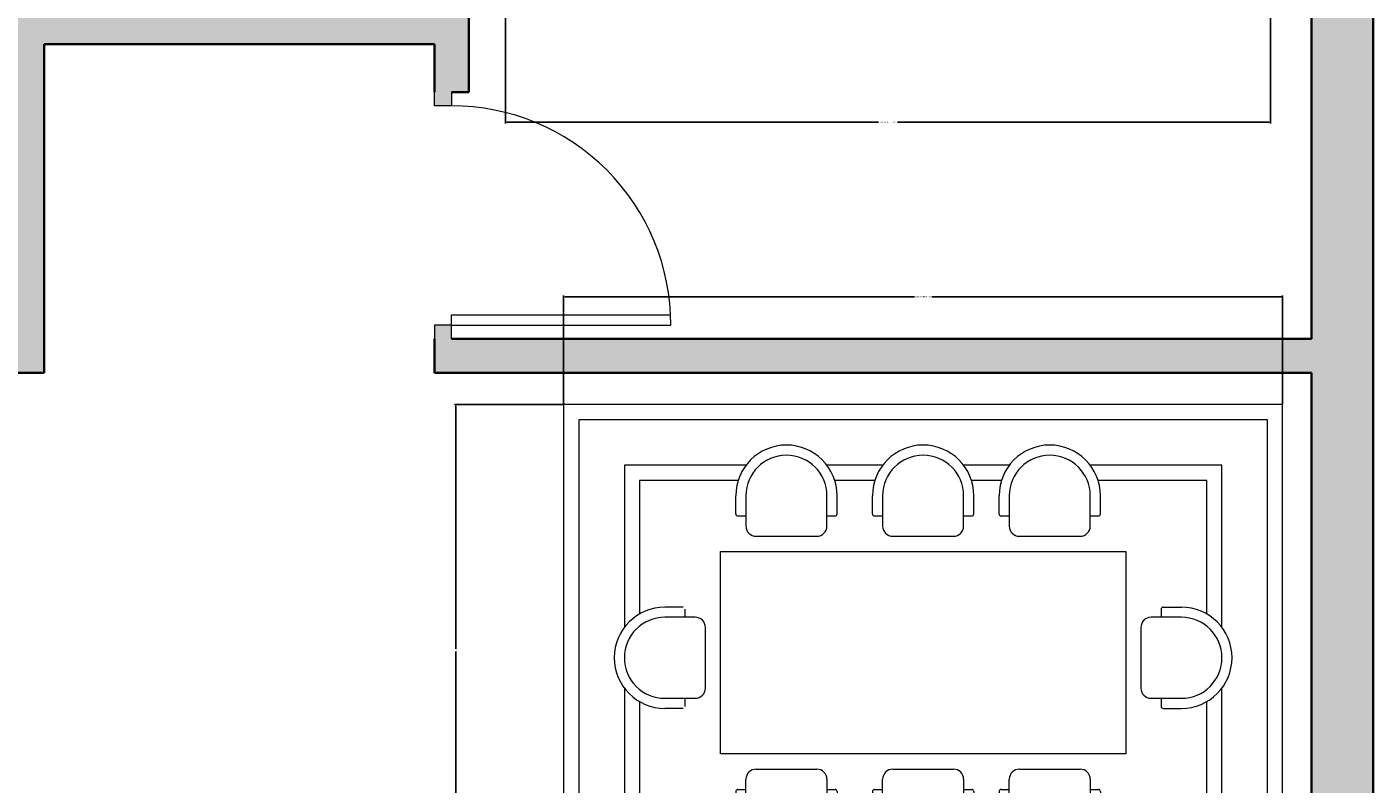
# Model space of a CAD drawing. Units: inches. Extents: x 2948 to 4025, y 2171 to 2966.
# Tile 4 of 6: x 3159 to 3356, y 2560 to 2670. Entities that reach past the tile are written whole.
import ezdxf

# ---------------------------------------------------------------- set-up
doc = ezdxf.new("R2010")
doc.units = ezdxf.units.IN
for name, color, linetype, lineweight in [('A-ANNO-DIMS', 2, 'Continuous', 18), ('A-DOOR', 3, 'Continuous', 18), ('A-FURN', 8, 'Continuous', 18), ('A-WALL', 7, 'Continuous', 35), ('A-WALL-PATT', 252, 'Continuous', 13)]:
    doc.layers.add(name, color=color, linetype=linetype, lineweight=lineweight)
doc.styles.get("Standard").update_dxf_attribs({"font": 'arial.ttf'})
doc.dimstyles.get("Standard").update_dxf_attribs({"dimtxt": 0.18, "dimasz": 0.18, "dimexe": 0.18, "dimexo": 0.0625, "dimgap": 0.09, "dimtad": 0, "dimtih": 1, "dimtoh": 1, "dimdec": 4, "dimzin": 0, "dimdsep": 46, "dimtxsty": 'Standard', "dimcen": 0.09, "dimadec": 0, "dimazin": 0, "dimtfac": 1, "dimtdec": 4, "dimtofl": 0, "dimtmove": 0, "dimatfit": 3, "dimfxl": 1, "dimtolj": 1, "dimtzin": 0, "dimarcsym": 0})

# ---------------------------------------------------------------- blocks, each defined once
blk = doc.blocks.new('A$C27801A2F')
for p, q in [((3.55, 2.425), (0, 2.425)), ((0, 2.425), (0, 0)), ((3.55, 0), (3.55, 2.425)), ((3.475, 2.35), (0.075, 2.35)), ((0.075, 2.35), (0.075, 0.075)), ((3.475, 0.075), (3.475, 2.35)), ((0.9, 2.125), (0.3, 2.125)), ((0.3, 2.125), (0.3, 1.325)), ((1.575, 2.125), (1.3, 2.125)), ((2.2, 2.125), (1.975, 2.125)), ((3.25, 2.125), (2.6, 2.125)), ((3.25, 1.325), (3.25, 2.125)), ((0.375, 2.05), (0.375, 1.3915)), ((0.8615, 2.05), (0.375, 2.05)), ((1.5365, 2.05), (1.3385, 2.05)), ((2.1615, 2.05), (2.0135, 2.05)), ((3.175, 2.05), (2.6385, 2.05)), ((3.175, 1.3915), (3.175, 2.05)), ((0.85, 1.885), (0.85, 1.975)), ((0.9, 1.975), (0.9, 1.825)), ((1.3, 1.825), (1.3, 1.975)), ((1.35, 1.885), (1.35, 1.975)), ((1.525, 1.885), (1.525, 1.975)), ((1.575, 1.975), (1.575, 1.825)), ((1.975, 1.825), (1.975, 1.975)), ((2.025, 1.885), (2.025, 1.975)), ((2.15, 1.885), (2.15, 1.975)), ((2.2, 1.975), (2.2, 1.825)), ((2.6, 1.825), (2.6, 1.975)), ((2.65, 1.885), (2.65, 1.975)), ((0.86, 1.875), (0.9, 1.875)), ((1.3, 1.875), (1.34, 1.875)), ((1.535, 1.875), (1.575, 1.875)), ((1.975, 1.875), (2.015, 1.875)), ((2.16, 1.875), (2.2, 1.875)), ((2.6, 1.875), (2.64, 1.875)), ((0.95, 1.775), (1.25, 1.775)), ((1.625, 1.775), (1.925, 1.775)), ((2.25, 1.775), (2.55, 1.775)), ((0.775, 0.7), (0.775, 1.7)), ((0.775, 1.7), (2.775, 1.7)), ((2.775, 1.7), (2.775, 0.7)), ((0.59, 1.425), (0.5, 1.425)), ((0.6, 1.375), (0.6, 1.415)), ((2.95, 1.415), (2.95, 1.375)), ((2.96, 1.425), (3.05, 1.425)), ((0.65, 1.375), (0.5, 1.375)), ((3.05, 1.375), (2.9, 1.375)), ((0.7, 1.025), (0.7, 1.325)), ((2.85, 1.325), (2.85, 1.025)), ((0.3, 1.025), (0.3, 0.275)), ((3.25, 0.275), (3.25, 1.025)), ((0.375, 0.9585), (0.375, 0.35)), ((0.5, 0.975), (0.65, 0.975)), ((0.6, 0.935), (0.6, 0.975)), ((2.9, 0.975), (3.05, 0.975)), ((2.95, 0.975), (2.95, 0.935)), ((3.175, 0.35), (3.175, 0.9585)), ((0.59, 0.925), (0.5, 0.925)), ((2.96, 0.925), (3.05, 0.925)), ((2.775, 0.7), (0.775, 0.7)), ((0.95, 0.625), (1.25, 0.625)), ((1.625, 0.625), (1.925, 0.625)), ((2.25, 0.625), (2.55, 0.625)), ((0.9, 0.425), (0.9, 0.575)), ((1.3, 0.575), (1.3, 0.425)), ((1.575, 0.425), (1.575, 0.575)), ((1.975, 0.575), (1.975, 0.425)), ((2.2, 0.425), (2.2, 0.575)), ((2.6, 0.575), (2.6, 0.425)), ((0.85, 0.515), (0.85, 0.425)), ((0.86, 0.525), (0.9, 0.525)), ((1.3, 0.525), (1.34, 0.525)), ((1.35, 0.515), (1.35, 0.425)), ((1.525, 0.515), (1.525, 0.425)), ((1.535, 0.525), (1.575, 0.525)), ((1.975, 0.525), (2.015, 0.525)), ((2.025, 0.515), (2.025, 0.425)), ((2.15, 0.515), (2.15, 0.425)), ((2.16, 0.525), (2.2, 0.525)), ((2.6, 0.525), (2.64, 0.525)), ((2.65, 0.515), (2.65, 0.425)), ((0.375, 0.35), (0.8615, 0.35)), ((1.3385, 0.35), (1.5365, 0.35)), ((2.0135, 0.35), (2.1615, 0.35)), ((2.6385, 0.35), (3.175, 0.35)), ((0.3, 0.275), (0.9, 0.275)), ((1.3, 0.275), (1.575, 0.275)), ((1.975, 0.275), (2.2, 0.275)), ((2.6, 0.275), (3.25, 0.275)), ((0.075, 0.075), (3.475, 0.075)), ((0, 0), (3.55, 0))]:
    blk.add_line(p, q)
for centre, radius, start, end in [((1.1, 1.975), 0.25, 0, 180), ((1.775, 1.975), 0.25, 0, 180), ((2.4, 1.975), 0.25, 0, 180), ((1.1, 1.975), 0.2, 0.00007, 179.99993), ((1.775, 1.975), 0.2, 0.00007, 179.99993), ((2.4, 1.975), 0.2, 0.00007, 179.99993), ((0.86, 1.885), 0.01, 180, 270), ((1.34, 1.885), 0.01, 270, 0), ((1.535, 1.885), 0.01, 180, 270), ((2.015, 1.885), 0.01, 270, 0), ((2.16, 1.885), 0.01, 180, 270), ((2.64, 1.885), 0.01, 270, 0), ((0.95, 1.825), 0.05, 180, 270), ((1.25, 1.825), 0.05, 270, 0), ((1.625, 1.825), 0.05, 180, 270), ((1.925, 1.825), 0.05, 270, 0), ((2.25, 1.825), 0.05, 180, 270), ((2.55, 1.825), 0.05, 270, 0), ((0.5, 1.175), 0.25, 90, 270), ((2.96, 1.415), 0.01, 90, 180), ((3.05, 1.175), 0.25, 270, 90), ((0.5, 1.175), 0.2, 90.00007, 269.99993), ((0.65, 1.325), 0.05, 0, 90), ((2.9, 1.325), 0.05, 90, 180), ((3.05, 1.175), 0.2, 270.00007, 89.99993), ((0.65, 1.025), 0.05, 270, 0), ((2.9, 1.025), 0.05, 180, 270), ((2.96, 0.935), 0.01, 180, 270), ((0.95, 0.575), 0.05, 90, 180), ((1.25, 0.575), 0.05, 0, 90), ((1.625, 0.575), 0.05, 90, 180), ((1.925, 0.575), 0.05, 0, 90), ((2.25, 0.575), 0.05, 90, 180), ((2.55, 0.575), 0.05, 0, 90), ((0.86, 0.515), 0.01, 90, 180), ((1.34, 0.515), 0.01, 0, 90), ((1.535, 0.515), 0.01, 90, 180), ((2.015, 0.515), 0.01, 0, 90), ((2.16, 0.515), 0.01, 90, 180), ((2.64, 0.515), 0.01, 0, 90), ((1.1, 0.425), 0.25, 180, 0), ((1.1, 0.425), 0.2, 180.00007, 359.99993), ((1.775, 0.425), 0.25, 180, 0), ((1.775, 0.425), 0.2, 180.00007, 359.99993), ((2.4, 0.425), 0.25, 180, 0), ((2.4, 0.425), 0.2, 180.00007, 359.99993)]:
    blk.add_arc(centre, radius, start, end)
blk = doc.blocks.new('DOOR-SWING-32IN')
for p, q in [((2, 34.5), (0, 34.5)), ((2, 32), (2, 34.5)), ((34, 32), (34, 34.5)), ((34, 34.5), (36, 34.5)), ((0, 32), (2, 32)), ((2, 32), (2, 0)), ((2, 32), (3.5, 32)), ((3.5, 32), (3.5, 0.04)), ((36, 32), (34, 32))]:
    blk.add_line(p, q)
blk.add_arc((2, 32), 32, 270, 0)
blk = doc.blocks.new('*D27')
at = {"layer": 'A-ANNO-DIMS', "color": 0, "lineweight": -2, "transparency": 16777216}
for p, q in [((3228.87, 2673.27), (3228.87, 2656.41)), ((3340.53, 2673.27), (3340.53, 2656.41)), ((3229.05, 2656.59), (3283.31, 2656.59)), ((3340.35, 2656.59), (3286.08, 2656.59))]:
    blk.add_line(p, q, dxfattribs=at)
at = {"layer": 'A-ANNO-DIMS', "color": 0, "transparency": 16777216}
for points in [[(3229.05, 2656.62), (3229.05, 2656.56), (3228.87, 2656.59)], [(3340.35, 2656.62), (3340.35, 2656.56), (3340.53, 2656.59)]]:
    blk.add_solid(points, dxfattribs=at)
at = {"layer": 'Defpoints', "color": 0, "transparency": 16777216}
for p in [(3228.87, 2673.34), (3340.53, 2673.34), (3340.53, 2656.59)]:
    blk.add_point(p, dxfattribs=at)
at = {"layer": 'A-ANNO-DIMS', "color": 0, "transparency": 16777216, "insert": (3284.7, 2656.59), "char_height": 0.18, "attachment_point": 5}
blk.add_mtext('\\A1;BED GROUP 112 TYP.', dxfattribs=at)
blk = doc.blocks.new('*D29')
at = {"layer": 'A-ANNO-DIMS', "color": 0, "lineweight": -2, "transparency": 16777216}
for p, q in [((3237.36, 2615.44), (3237.36, 2631.3)), ((3342.31, 2615.44), (3342.31, 2631.3)), ((3237.54, 2631.12), (3288.58, 2631.12)), ((3342.13, 2631.12), (3291.09, 2631.12))]:
    blk.add_line(p, q, dxfattribs=at)
at = {"layer": 'A-ANNO-DIMS', "color": 0, "transparency": 16777216}
for points in [[(3237.54, 2631.15), (3237.54, 2631.09), (3237.36, 2631.12)], [(3342.13, 2631.15), (3342.13, 2631.09), (3342.31, 2631.12)]]:
    blk.add_solid(points, dxfattribs=at)
at = {"layer": 'Defpoints', "color": 0, "transparency": 16777216}
for p in [(3342.31, 2631.12), (3237.36, 2615.38), (3342.31, 2615.38)]:
    blk.add_point(p, dxfattribs=at)
at = {"layer": 'A-ANNO-DIMS', "color": 0, "transparency": 16777216, "insert": (3289.84, 2631.12), "char_height": 0.18, "attachment_point": 5}
blk.add_mtext('\\A1;DINING GROUP 105', dxfattribs=at)
blk = doc.blocks.new('*D30')
at = {"layer": 'A-ANNO-DIMS', "color": 0, "lineweight": -2, "transparency": 16777216}
for p, q in [((3237.3, 2615.38), (3221.43, 2615.38)), ((3221.61, 2615.2), (3221.61, 2579.71)), ((3221.61, 2543.86), (3221.61, 2579.35)), ((3237.3, 2543.68), (3221.43, 2543.68))]:
    blk.add_line(p, q, dxfattribs=at)
at = {"layer": 'A-ANNO-DIMS', "color": 0, "transparency": 16777216}
for points in [[(3221.58, 2615.2), (3221.64, 2615.2), (3221.61, 2615.38)], [(3221.58, 2543.86), (3221.64, 2543.86), (3221.61, 2543.68)]]:
    blk.add_solid(points, dxfattribs=at)
at = {"layer": 'Defpoints', "color": 0, "transparency": 16777216}
for p in [(3221.61, 2615.38), (3237.36, 2615.38), (3237.36, 2543.68)]:
    blk.add_point(p, dxfattribs=at)
at = {"layer": 'A-ANNO-DIMS', "color": 0, "transparency": 16777216, "insert": (3221.61, 2579.53), "char_height": 0.18, "attachment_point": 5}
blk.add_mtext('\\A1;72', dxfattribs=at)
blk = doc.blocks.new('*D38')
at = {"layer": 'A-ANNO-DIMS', "color": 0, "lineweight": -2, "transparency": 16777216}
for p, q in [((2979.45, 2777.99), (2948.13, 2777.99)), ((2948.31, 2777.81), (2948.31, 2507.17)), ((2948.31, 2236.17), (2948.31, 2506.8)), ((3217.45, 2235.99), (2948.13, 2235.99))]:
    blk.add_line(p, q, dxfattribs=at)
at = {"layer": 'A-ANNO-DIMS', "color": 0, "transparency": 16777216}
for points in [[(2948.28, 2777.81), (2948.34, 2777.81), (2948.31, 2777.99)], [(2948.28, 2236.17), (2948.34, 2236.17), (2948.31, 2235.99)]]:
    blk.add_solid(points, dxfattribs=at)
at = {"layer": 'Defpoints', "color": 0, "transparency": 16777216}
for p in [(2948.31, 2777.99), (2979.51, 2777.99), (3217.51, 2235.99)]:
    blk.add_point(p, dxfattribs=at)
at = {"layer": 'A-ANNO-DIMS', "color": 0, "transparency": 16777216, "insert": (2948.31, 2506.99), "char_height": 0.18, "attachment_point": 5}
blk.add_mtext('\\A1;542', dxfattribs=at)

msp = doc.modelspace()

# ---------------------------------------------------------------- hatches: boundary and pattern name
at = {"layer": 'A-WALL-PATT'}
h = msp.add_hatch(color=256, dxfattribs=at)
h.dxf.hatch_style = 1
h.paths.add_polyline_path([(3178.0136, 2777.9862), (3108.5136, 2777.9862), (3108.5136, 2768.9862), (3156.5136, 2768.9862), (3156.5136, 2624.9862), (3132.5136, 2624.9862), (3130.5136, 2624.9862), (3130.5136, 2622.4862), (3132.5136, 2622.4862), (3132.5136, 2619.9862), (3161.5136, 2619.9862), (3161.5136, 2667.9862), (3218.5136, 2667.9862), (3218.5136, 2660.9862), (3218.5136, 2658.9862), (3221.0136, 2658.9862), (3221.0136, 2660.9862), (3223.5136, 2660.9862), (3223.5136, 2676.9862), (3221.0136, 2676.9862), (3221.0136, 2678.9862), (3218.5136, 2678.9862), (3218.5136, 2676.9862), (3218.5136, 2672.9862), (3161.5136, 2672.9862), (3161.5136, 2768.9862), (3178.0136, 2768.9862)])
h = msp.add_hatch(color=256, dxfattribs=at)
h.dxf.hatch_style = 1
h.paths.add_polyline_path([(3355.5136, 2777.9862), (3321.0136, 2777.9862), (3321.0136, 2768.9862), (3346.5136, 2768.9862), (3346.5136, 2624.9862), (3221.0136, 2624.9862), (3221.0136, 2626.9862), (3218.5136, 2626.9862), (3218.5136, 2624.9862), (3218.5136, 2619.9862), (3346.5136, 2619.9862), (3346.5136, 2517.9862), (3355.5136, 2517.9862)])

# ---------------------------------------------------------------- linework, layer by layer
at = {"layer": 'A-DOOR'}
msp.add_line((3221.0136, 2626.9862), (3221.0136, 2626.9862), dxfattribs=at)
at = {"layer": 'A-WALL'}
for p, q in [((3355.5136, 2777.9862), (3355.5136, 2235.9862)), ((3346.5136, 2768.9862), (3346.5136, 2624.9862)), ((3223.5136, 2676.9862), (3223.5136, 2660.9862)), ((3161.5136, 2667.9862), (3218.5136, 2667.9862)), ((3161.5136, 2667.9862), (3161.5136, 2619.9862)), ((3218.5136, 2667.9862), (3218.5136, 2660.9862)), ((3221.0136, 2660.9862), (3223.5136, 2660.9862)), ((3218.5136, 2624.9862), (3218.5136, 2619.9862)), ((3221.0136, 2624.9862), (3346.5136, 2624.9862)), ((3132.5136, 2619.9862), (3161.5136, 2619.9862)), ((3218.5136, 2619.9862), (3346.5136, 2619.9862)), ((3346.5136, 2619.9862), (3346.5136, 2343.9862))]:
    msp.add_line(p, q, dxfattribs=at)

# ---------------------------------------------------------------- block references
at = {"layer": 'A-DOOR', "rotation": 90.00000000000416}
msp.add_blockref('DOOR-SWING-32IN', (3253.0139, 2624.9866), dxfattribs=at)
at = {"layer": 'A-FURN', "xscale": 29.56530689526184, "yscale": 29.56530689526184, "zscale": 29.56530689526184}
msp.add_blockref('A$C27801A2F', (3237.3577, 2543.681), dxfattribs=at)

# ---------------------------------------------------------------- dimensions: what is measured, and where the dimension line sits
at = {"layer": 'A-ANNO-DIMS'}
for base, p1, p2, picture, middle in [((2948.3136, 2777.9862), (3217.5136, 2235.9862), (2979.5136, 2777.9862), '*D38', (2948.3136, 2506.9862)), ((3221.6141, 2615.3768), (3237.3577, 2543.681), (3237.3577, 2615.3768), '*D30', (3221.6141, 2579.5289))]:
    dim = msp.add_linear_dim(base=base, p1=p1, p2=p2, angle=90, dimstyle='Standard', override={"dimdec": 0, "dimlfac": 1, "dimrnd": 0, "dimzin": 0, "dimdsep": 46, "dimlunit": 2}, dxfattribs=at)
    dim.commit()
    dim.dimension.update_dxf_attribs({"geometry": picture, "text_midpoint": middle})
for base, p1, p2, text, picture, middle in [((3340.5311, 2656.5867), (3228.8657, 2673.3365), (3340.5311, 2673.3365), 'BED GROUP <> TYP.', '*D27', (3284.6984, 2656.5867)), ((3342.3145, 2631.1204), (3237.3577, 2615.3768), (3342.3145, 2615.3768), 'DINING GROUP <>', '*D29', (3289.8361, 2631.1204))]:
    dim = msp.add_linear_dim(base=base, p1=p1, p2=p2, text=text, dimstyle='Standard', override={"dimdec": 0, "dimlfac": 1, "dimrnd": 0, "dimzin": 0, "dimdsep": 46, "dimlunit": 2}, dxfattribs=at)
    dim.commit()
    dim.dimension.update_dxf_attribs({"geometry": picture, "text_midpoint": middle})

doc.saveas('drawing.dxf')
